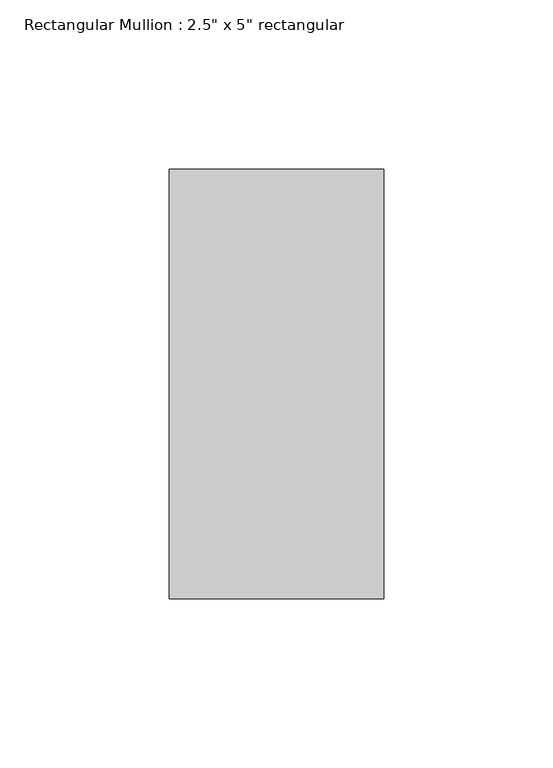
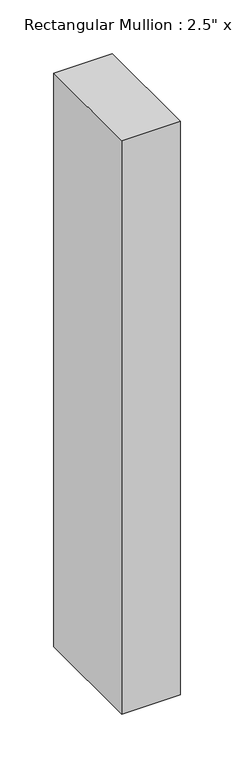
"""IFC4 building model written with IfcOpenShell, lengths in millimetres: member geometry."""

from ifc_helpers import new_model, si_unit, frame, origin, place, context, project, spatial, polyline, outline, extrude, source, transform, mapped, element, save


def member_a044dc63(model_context):
    return source(origin(), model_context, "Body", "SweptSolid", [
        extrude(outline(polyline([(0.0, 63.5), (0.0, -63.5), (-63.5, -63.5), (-63.5, 63.5), (0.0, 63.5)])), frame((0.0, 0.0, -654.1955358), z_axis=(0.0, 0.0, 1.0), x_axis=(1.0, 0.0, 0.0)), (0.0, 0.0, 1.0), 654.1955358),
    ])


if __name__ == "__main__":
    model = new_model("IFC4")
    model_context = context("Model", 3, world=origin())
    ifc_project = project(units=[si_unit("LENGTHUNIT", "METRE", prefix="MILLI")], contexts=[model_context])
    site = spatial("IfcSite", under=ifc_project)
    building = spatial("IfcBuilding", under=site)
    placement = place(None, origin())
    member_shape = member_a044dc63(model_context)
    element("IfcMember", 1, ObjectType="Rectangular Mullion : 2.5\" x 5\" rectangular", at=placement, inside=building, context=model_context, shape_type="MappedRepresentation", body=[
        mapped(member_shape, transform((0.0, 0.0, 0.0), x_axis=(1.0, 0.0, 0.0), y_axis=(0.0, 1.0, 0.0), z_axis=(0.0, 0.0, 1.0))),
    ])
    save(model, "model.ifc")

# Revit data of these elements
# Type "Rectangular Mullion : 2.5\" x 5\" rectangular"
#   built-in parameter 1007304 = 0.416667 (stored number, unit not read)
#   built-in parameter 1007301 = 0.104167 (stored number, unit not read)
#   built-in parameter 1007300 = 0.104167 (stored number, unit not read)
# Element 1 (IfcMember, "Rectangular Mullion : 2.5\" x 5\" rectangular")
#   Materials on its faces: "Aluminum"
# Materials
#   "Aluminum": class "Metal", colour RGB 247 247 247, transparency 0, Description = "Aluminum 6061", Cost = 0
